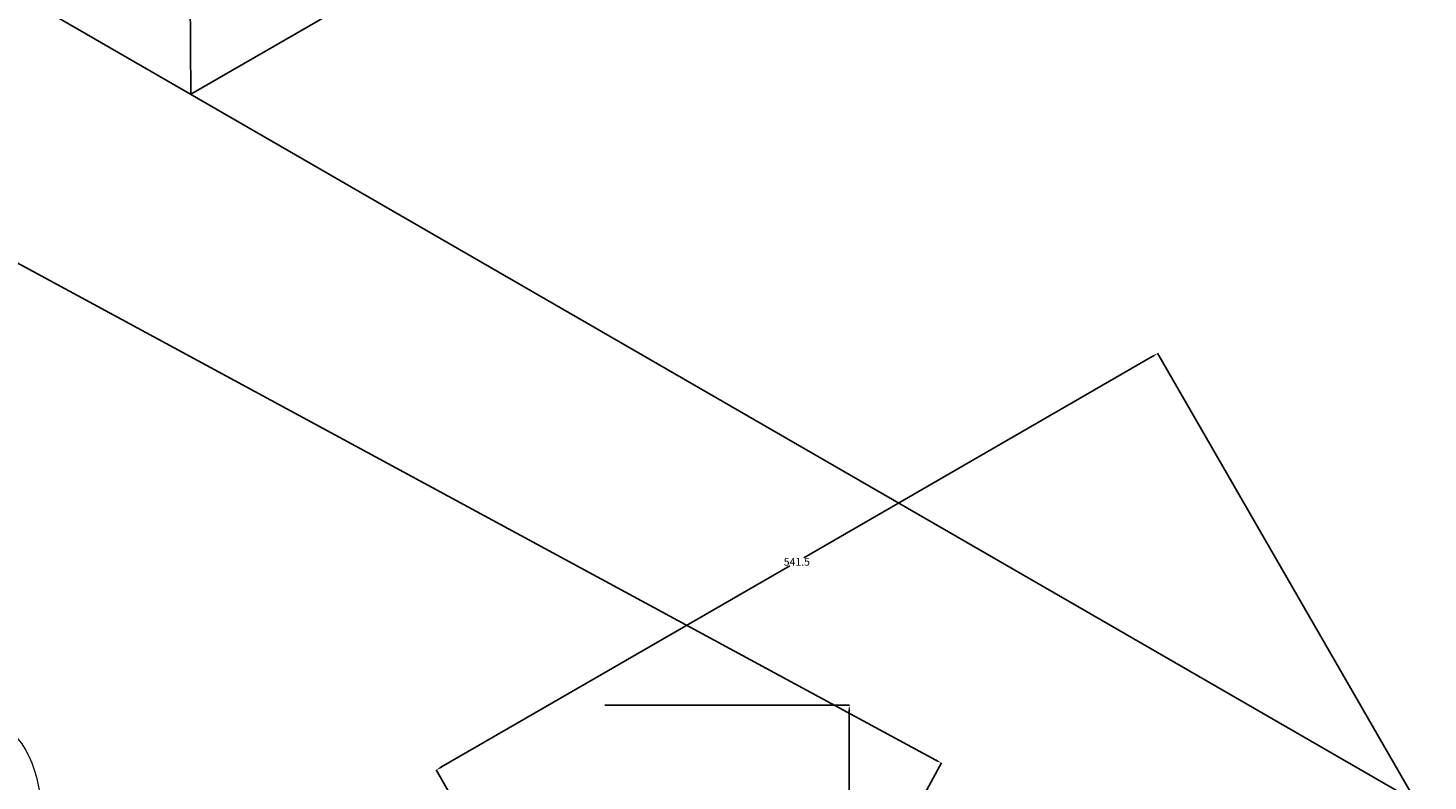
# Model space of a CAD drawing. Units: metres. Extents: x -2391 to 4922, y -635 to 4845.
# Tile 10 of 37: x -871 to 39, y 919 to 1408. Entities that reach past the tile are written whole.
import ezdxf

# ---------------------------------------------------------------- set-up
doc = ezdxf.new("R2010")
doc.units = ezdxf.units.M
doc.header["$MEASUREMENT"] = 0
for name, color, linetype, lineweight in [('A-ANNO-DIMS', 2, 'Continuous', 18), ('A-FLOR-FIXT', 3, 'Continuous', 25), ('A-FURN', 8, 'Continuous', 18)]:
    doc.layers.add(name, color=color, linetype=linetype, lineweight=lineweight)
doc.styles.get("Standard").update_dxf_attribs({"font": 'arial.ttf'})
doc.dimstyles.get("Standard").update_dxf_attribs({"dimtxt": 5, "dimasz": 4, "dimexe": 0.18, "dimexo": 0.0625, "dimgap": 0.09, "dimtad": 0, "dimtih": 1, "dimtoh": 1, "dimdec": 0, "dimzin": 0, "dimdsep": 46, "dimtxsty": 'Standard', "dimcen": 0.09, "dimadec": 0, "dimazin": 0, "dimtfac": 1, "dimtdec": 0, "dimtofl": 0, "dimtmove": 0, "dimatfit": 3, "dimfxl": 1, "dimtolj": 1, "dimtzin": 0, "dimarcsym": 0})

# ---------------------------------------------------------------- blocks, each defined once
blk = doc.blocks.new('STOOL-BAR')
for p, q in [((193.66, 114.21), (193.66, 537.32)), ((227.15, 541.57), (227.15, 114.21))]:
    blk.add_line(p, q)
blk.add_arc((210.41, 114.21), 16.75, 180, 0)
for points, knots in [([(47.24, 931.27), (26.82, 772.78), (-15.55, 443.76), (639.86, 614.21), (403.75, 766.18), (59.87, 548.32), (308.37, 1061.03), (87.86, 1049.28), (63.7, 979.1), (47.24, 931.27)], [0, 0, 0, 0, 373.373325, 775.091582, 839.205201, 1103.589215, 1452.822506, 1516.235646, 1651.960559, 1651.960559, 1651.960559, 1651.960559]), ([(82.71, 605.1), (79.37, 599.07), (25.39, 501.43), (205.15, 535.32), (373.81, 567.12)], [0, 0, 0, 0, 19.816883, 320.720948, 320.720948, 320.720948, 320.720948]), ([(193.66, 199.14), (106.89, 200.34), (-113.88, 203.37), (215.44, -95.9), (508.37, 143.53), (296.52, 208.79), (227.15, 200.77)], [0, 0, 0, 0, 131.596892, 334.838301, 476.929251, 613.088937, 613.088937, 613.088937, 613.088937])]:
    blk.add_open_spline(points, degree=3, knots=knots)
blk = doc.blocks.new('*D6')
at = {"layer": 'A-ANNO-DIMS', "color": 0, "lineweight": -2, "transparency": 16777216}
for p, q in [((-496.54, 968.1), (-337.38, 968.1)), ((-337.56, 964.1), (-337.56, 440.64)), ((-337.56, -88.18), (-337.56, 435.28)), ((-496.54, -92.18), (-337.38, -92.18))]:
    blk.add_line(p, q, dxfattribs=at)
at = {"layer": 'A-ANNO-DIMS', "color": 0, "transparency": 16777216}
for points in [[(-338.23, 964.1), (-336.89, 964.1), (-337.56, 968.1)], [(-338.23, -88.18), (-336.89, -88.18), (-337.56, -92.18)]]:
    blk.add_solid(points, dxfattribs=at)
at = {"layer": 'Defpoints', "color": 0, "transparency": 16777216}
for p in [(-496.6, 968.1), (-337.56, 968.1), (-496.6, -92.18)]:
    blk.add_point(p, dxfattribs=at)
at = {"layer": 'A-ANNO-DIMS', "color": 0, "transparency": 16777216, "insert": (-337.56, 437.96), "char_height": 5, "attachment_point": 5}
blk.add_mtext('\\A1;BAR STOOL 1060 TYP.', dxfattribs=at)
blk = doc.blocks.new('*D8')
at = {"layer": 'A-ANNO-DIMS', "color": 0, "lineweight": -2, "transparency": 16777216}
for p, q in [((-2047.33, 3005.21), (-2047.33, -631.4)), ((4577.76, 2350.21), (4577.76, -631.4)), ((-2043.33, -631.22), (1257.62, -631.22)), ((4573.76, -631.22), (1272.8, -631.22))]:
    blk.add_line(p, q, dxfattribs=at)
at = {"layer": 'A-ANNO-DIMS', "color": 0, "transparency": 16777216}
for points in [[(-2043.33, -630.56), (-2043.33, -631.89), (-2047.33, -631.22)], [(4573.76, -630.56), (4573.76, -631.89), (4577.76, -631.22)]]:
    blk.add_solid(points, dxfattribs=at)
at = {"layer": 'Defpoints', "color": 0, "transparency": 16777216}
for p in [(-2047.33, 3005.28), (4577.76, 2350.28), (4577.76, -631.22)]:
    blk.add_point(p, dxfattribs=at)
at = {"layer": 'A-ANNO-DIMS', "color": 0, "transparency": 16777216, "insert": (1265.21, -631.22), "char_height": 5, "attachment_point": 5}
blk.add_mtext('\\A1;6625', dxfattribs=at)
blk = doc.blocks.new('*D10')
at = {"layer": 'A-ANNO-DIMS', "color": 0, "lineweight": -2, "transparency": 16777216}
for p, q in [((550.68, 4505.28), (-2384.01, 4505.28)), ((-2383.83, 4501.28), (-2383.83, 2107.92)), ((-2383.83, -290.72), (-2383.83, 2102.63)), ((-488.55, -294.72), (-2384.01, -294.72))]:
    blk.add_line(p, q, dxfattribs=at)
at = {"layer": 'A-ANNO-DIMS', "color": 0, "transparency": 16777216}
for points in [[(-2384.5, 4501.28), (-2383.17, 4501.28), (-2383.83, 4505.28)], [(-2384.5, -290.72), (-2383.17, -290.72), (-2383.83, -294.72)]]:
    blk.add_solid(points, dxfattribs=at)
at = {"layer": 'Defpoints', "color": 0, "transparency": 16777216}
for p in [(-2383.83, 4505.28), (550.74, 4505.28), (-488.49, -294.72)]:
    blk.add_point(p, dxfattribs=at)
at = {"layer": 'A-ANNO-DIMS', "color": 0, "transparency": 16777216, "insert": (-2383.83, 2105.28), "char_height": 5, "attachment_point": 5}
blk.add_mtext('\\A1;4800', dxfattribs=at)
blk = doc.blocks.new('*D46')
at = {"layer": 'A-ANNO-DIMS', "color": 0, "lineweight": -2, "transparency": 16777216}
for p, q in [((-2047.3, 1505.33), (-1887.13, 1801.4)), ((-1883.7, 1799.34), (-1087.36, 1368.5)), ((-281.24, 932.38), (-1077.58, 1363.21)), ((-437.81, 634.57), (-277.64, 930.64))]:
    blk.add_line(p, q, dxfattribs=at)
at = {"layer": 'A-ANNO-DIMS', "color": 0, "transparency": 16777216}
for points in [[(-1883.38, 1799.92), (-1884.01, 1798.75), (-1887.21, 1801.24)], [(-280.92, 932.97), (-281.56, 931.8), (-277.72, 930.48)]]:
    blk.add_solid(points, dxfattribs=at)
at = {"layer": 'Defpoints', "color": 0, "transparency": 16777216}
for p in [(-2047.33, 1505.28), (-277.72, 930.48), (-437.84, 634.52)]:
    blk.add_point(p, dxfattribs=at)
at = {"layer": 'A-ANNO-DIMS', "color": 0, "transparency": 16777216, "insert": (-1082.47, 1365.86), "char_height": 5, "attachment_point": 5}
blk.add_mtext('\\A1;1830', dxfattribs=at)
blk = doc.blocks.new('*D47')
at = {"layer": 'A-ANNO-DIMS', "color": 0, "lineweight": -2, "transparency": 16777216}
for p, q in [((-140.59, 1194.69), (-367.03, 1063.96)), ((31.1, 905.33), (-137.21, 1196.85)), ((-602.63, 927.94), (-376.18, 1058.67)), ((-437.87, 634.57), (-606.18, 926.09))]:
    blk.add_line(p, q, dxfattribs=at)
at = {"layer": 'A-ANNO-DIMS', "color": 0, "transparency": 16777216}
for points in [[(-140.92, 1195.27), (-140.25, 1194.12), (-137.12, 1196.69)], [(-602.96, 928.51), (-602.29, 927.36), (-606.09, 925.94)]]:
    blk.add_solid(points, dxfattribs=at)
at = {"layer": 'Defpoints', "color": 0, "transparency": 16777216}
for p in [(-137.12, 1196.69), (31.13, 905.28), (-437.84, 634.52)]:
    blk.add_point(p, dxfattribs=at)
at = {"layer": 'A-ANNO-DIMS', "color": 0, "transparency": 16777216, "insert": (-371.61, 1061.31), "char_height": 5, "attachment_point": 5}
blk.add_mtext('\\A1;541.5', dxfattribs=at)

msp = doc.modelspace()

# ---------------------------------------------------------------- linework, layer by layer
at = {"layer": 'A-FLOR-FIXT'}
for p, q in [((-771.7543, 2188.8198), (-765.6167, 1365.2763)), ((550.7419, 2125.2763), (-765.6167, 1365.2763)), ((-1527.7191, 1805.2763), (31.1266, 905.2763))]:
    msp.add_line(p, q, dxfattribs=at)

# ---------------------------------------------------------------- block references
at = {"layer": 'A-FURN'}
msp.add_blockref('STOOL-BAR', (-1086.3941, -85.4426), dxfattribs=at)

# ---------------------------------------------------------------- dimensions: what is measured, and where the dimension line sits
at = {"layer": 'A-ANNO-DIMS'}
for base, p1, p2, angle, override, picture, middle in [((-2383.8343, 4505.2763), (-488.4886, -294.7237), (550.7419, 4505.2763), 90, {"dimdec": 0, "dimlfac": 1, "dimrnd": 0, "dimzin": 0, "dimdsep": 46, "dimlunit": 2}, '*D10', (-2383.8343, 2105.2763)), ((-277.7211, 930.4802), (-2047.3343, 1505.2763), (-437.841, 634.5176), 331.5859855, {"dimdec": 0, "dimlfac": 1, "dimrnd": 0, "dimzin": 0, "dimdsep": 46, "dimlunit": 2}, '*D46', (-1082.4677, 1365.8595)), ((-137.1234, 1196.6938), (-437.841, 634.5176), (31.1266, 905.2763), 30, {"dimdec": 1, "dimlfac": 1, "dimrnd": 0, "dimzin": 0, "dimdsep": 46, "dimlunit": 2}, '*D47', (-371.6072, 1061.3145))]:
    dim = msp.add_linear_dim(base=base, p1=p1, p2=p2, angle=angle, dimstyle='Standard', override=override, dxfattribs=at)
    dim.commit()
    dim.dimension.update_dxf_attribs({"geometry": picture, "text_midpoint": middle})
dim = msp.add_linear_dim(base=(4577.76, -631.2237), p1=(-2047.3343, 3005.2763), p2=(4577.76, 2350.2763), dimstyle='Standard', override={"dimdec": 0, "dimlfac": 1, "dimrnd": 0, "dimzin": 0, "dimdsep": 46, "dimlunit": 2}, dxfattribs=at)
dim.commit()
dim.dimension.update_dxf_attribs({"geometry": '*D8', "text_midpoint": (1265.2128, -631.2237)})
dim = msp.add_linear_dim(base=(-337.5616, 968.1038), p1=(-496.6042, -92.1799), p2=(-496.6042, 968.1038), angle=90, text='BAR STOOL <> TYP.', dimstyle='Standard', override={"dimdec": 0, "dimrnd": 0, "dimzin": 0, "dimlunit": 2}, dxfattribs=at)
dim.commit()
dim.dimension.update_dxf_attribs({"geometry": '*D6', "text_midpoint": (-337.5616, 437.9619)})

doc.saveas('drawing.dxf')
